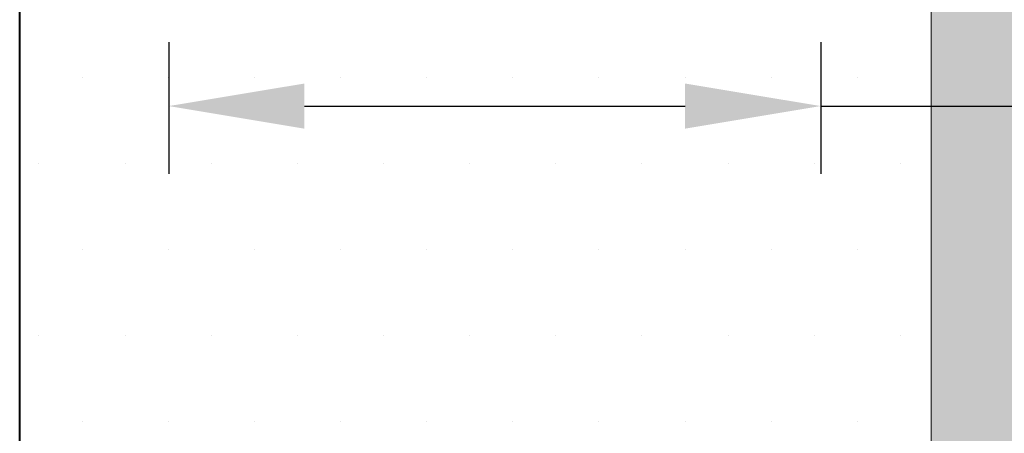
# Model space of a CAD drawing. Units: inches. Extents: x 459864 to 460310, y 324185 to 324787.
# Tile 3 of 112: x 460061 to 460079, y 324221 to 324229. Entities that reach past the tile are written whole.
import ezdxf

# ---------------------------------------------------------------- set-up
doc = ezdxf.new("R2010")
doc.units = ezdxf.units.IN
for name, color, linetype, lineweight in [('A-ANNO-DIMS', 2, 'Continuous', 18), ('A-WALL', 7, 'Continuous', 40), ('L-HRDS', 9, 'Continuous', 18), ('L-SITE-PATT', 252, 'Continuous', 13)]:
    doc.layers.add(name, color=color, linetype=linetype, lineweight=lineweight)
doc.styles.get("Standard").update_dxf_attribs({"font": 'arial.ttf'})
doc.dimstyles.new('ISO-25', dxfattribs={"dimtxt": 6, "dimasz": 2.5, "dimexe": 1.25, "dimexo": 0.625, "dimtad": 1, "dimdec": 1, "dimlunit": 3, "dimtxsty": 'Standard', "dimcen": 2.5, "dimadec": 0, "dimazin": 0, "dimtfac": 1, "dimtdec": 1, "dimtmove": 0, "dimatfit": 3, "dimfxl": 1, "dimarcsym": 0})

# ---------------------------------------------------------------- blocks, each defined once
blk = doc.blocks.new('*D36')
at = {"layer": 'A-ANNO-DIMS', "color": 0, "lineweight": -2, "transparency": 16777216}
for p, q in [((460063.861, 324228.483), (460063.861, 324226.056)), ((460075.876, 324228.483), (460075.876, 324226.056)), ((460066.361, 324227.306), (460073.376, 324227.306)), ((460075.876, 324227.306), (460126.021, 324227.306))]:
    blk.add_line(p, q, dxfattribs=at)
at = {"layer": 'A-ANNO-DIMS', "color": 0, "transparency": 16777216}
for points in [[(460066.361, 324227.722), (460066.361, 324226.889), (460063.861, 324227.306)], [(460073.376, 324227.722), (460073.376, 324226.889), (460075.876, 324227.306)]]:
    blk.add_solid(points, dxfattribs=at)
at = {"layer": 'Defpoints', "color": 0, "transparency": 16777216}
for p in [(460063.861, 324229.108), (460075.876, 324229.108), (460075.876, 324227.306)]:
    blk.add_point(p, dxfattribs=at)
at = {"layer": 'A-ANNO-DIMS', "color": 0, "transparency": 16777216, "insert": (460102.199, 324230.994), "char_height": 6, "attachment_point": 5}
blk.add_mtext('PAVER 1\'-0"', dxfattribs=at)

msp = doc.modelspace()

# ---------------------------------------------------------------- hatches: boundary and pattern name
at = {"layer": 'L-SITE-PATT'}
h = msp.add_hatch(dxfattribs=at)
h.set_pattern_fill('DOTS', color=256)
h.paths.add_polyline_path([(460269.804, 324283.483), (460247.115, 324283.483), (460121.929, 324283.483), (460121.929, 324252.473), (460117.429, 324252.473), (460110.124, 324252.473), (460110.124, 324243.287), (460080.83, 324243.287), (460080.83, 324252.473), (460061.115, 324252.473), (460061.115, 324251.882), (460077.909, 324251.882), (460077.909, 324199.483), (460080.83, 324199.483), (460080.83, 324207.553), (460110.124, 324207.553), (460110.124, 324199.483), (460110.813, 324199.483), (460262.115, 324199.483), (460269.804, 324199.483)], flags=17)
edge = h.paths.add_edge_path(flags=0)
edge.add_ellipse((460222.59, 324263.813), major_axis=(-8.485, 8.485), ratio=1, start_angle=405, end_angle=495, ccw=False)
edge.add_line((460214.821, 324254.66), (460214.832, 324254.666))
edge.add_ellipse((460222.59, 324263.813), major_axis=(-8.485, 8.485), ratio=1, start_angle=405, end_angle=495, ccw=False)
edge.add_line((460210.759, 324261.781), (460210.768, 324261.787))
edge.add_ellipse((460222.59, 324263.813), major_axis=(-8.485, 8.485), ratio=1, start_angle=405, end_angle=495, ccw=False)
edge.add_ellipse((460222.59, 324263.813), major_axis=(-8.485, 8.485), ratio=1, start_angle=392.754, end_angle=405, ccw=False)
edge.add_ellipse((460222.59, 324263.813), major_axis=(-8.485, 8.485), ratio=1, start_angle=380.9347, end_angle=392.754, ccw=False)
edge.add_line((460211.337, 324267.985), (460211.34, 324267.985))
edge.add_ellipse((460222.59, 324263.813), major_axis=(-8.485, 8.485), ratio=1, start_angle=380.9347, end_angle=392.754, ccw=False)
edge.add_ellipse((460222.59, 324263.813), major_axis=(-8.485, 8.485), ratio=1, start_angle=347.9015, end_angle=380.9347, ccw=False)
edge.add_ellipse((460222.59, 324263.813), major_axis=(-8.485, 8.485), ratio=1, start_angle=327.0619, end_angle=347.9015, ccw=False)
edge.add_ellipse((460222.59, 324263.813), major_axis=(-8.485, 8.485), ratio=1, start_angle=278.3246, end_angle=327.0619, ccw=False)
edge.add_line((460225.158, 324275.536), (460225.158, 324275.535))
edge.add_ellipse((460222.59, 324263.813), major_axis=(-8.485, 8.485), ratio=1, start_angle=278.3246, end_angle=327.0619, ccw=False)
edge.add_ellipse((460222.59, 324263.813), major_axis=(-8.485, 8.485), ratio=1, start_angle=260.6436, end_angle=278.3246, ccw=False)
edge.add_ellipse((460222.59, 324263.813), major_axis=(-8.485, 8.485), ratio=1, start_angle=225, end_angle=260.6436, ccw=False)
edge.add_line((460234.509, 324265.243), (460234.501, 324265.239))
edge.add_ellipse((460222.59, 324263.813), major_axis=(-8.485, 8.485), ratio=1, start_angle=225, end_angle=260.6436, ccw=False)
edge.add_ellipse((460222.59, 324263.813), major_axis=(-8.485, 8.485), ratio=1, start_angle=495, end_angle=585, ccw=False)
edge.add_line((460234.437, 324261.861), (460234.424, 324261.858))
edge.add_ellipse((460222.59, 324263.813), major_axis=(-8.485, 8.485), ratio=1, start_angle=495, end_angle=585, ccw=False)
edge.add_line((460227.95, 324253.067), (460227.946, 324253.083))
edge.add_ellipse((460222.59, 324263.813), major_axis=(-8.485, 8.485), ratio=1, start_angle=495, end_angle=585, ccw=False)
edge.add_line((460226.223, 324252.369), (460226.211, 324252.38))
edge.add_ellipse((460222.59, 324263.813), major_axis=(-8.485, 8.485), ratio=1, start_angle=495, end_angle=585, ccw=False)
h.paths.add_polyline_path([(460219.651, 324254.347), (460218.461, 324253.545), (460218.275, 324254.789), (460219.642, 324256.542), (460219.625, 324260.848), (460216.11, 324257.333), (460214.35, 324256.978), (460215.416, 324259.356), (460212.524, 324258.496), (460213.137, 324259.93), (460218.507, 324263.813), (460222.59, 324263.813), (460222.59, 324267.807), (460218.176, 324272.212), (460219.026, 324274.639), (460222.59, 324272.811), (460222.59, 324275.423), (460223.057, 324274.825), (460222.675, 324273.492), (460225.912, 324267.135), (460219.625, 324260.848)], flags=0)
edge = h.paths.add_edge_path(flags=0)
edge.add_ellipse((460194.576, 324264.046), major_axis=(-8.485, 8.485), ratio=1, start_angle=495, end_angle=585, ccw=False)
edge.add_line((460199.936, 324253.3), (460199.932, 324253.316))
edge.add_ellipse((460194.576, 324264.046), major_axis=(-8.485, 8.485), ratio=1, start_angle=495, end_angle=585, ccw=False)
edge.add_line((460198.208, 324252.603), (460198.196, 324252.613))
edge.add_ellipse((460194.576, 324264.046), major_axis=(-8.485, 8.485), ratio=1, start_angle=495, end_angle=585, ccw=False)
edge.add_ellipse((460194.576, 324264.046), major_axis=(-8.485, 8.485), ratio=1, start_angle=405, end_angle=495, ccw=False)
edge.add_line((460186.806, 324254.893), (460186.817, 324254.899))
edge.add_ellipse((460194.576, 324264.046), major_axis=(-8.485, 8.485), ratio=1, start_angle=405, end_angle=495, ccw=False)
edge.add_line((460182.744, 324262.014), (460182.753, 324262.02))
edge.add_ellipse((460194.576, 324264.046), major_axis=(-8.485, 8.485), ratio=1, start_angle=405, end_angle=495, ccw=False)
edge.add_ellipse((460194.576, 324264.046), major_axis=(-8.485, 8.485), ratio=1, start_angle=392.754, end_angle=405, ccw=False)
edge.add_ellipse((460194.576, 324264.046), major_axis=(-8.485, 8.485), ratio=1, start_angle=380.9347, end_angle=392.754, ccw=False)
edge.add_line((460183.323, 324268.218), (460183.326, 324268.218))
edge.add_ellipse((460194.576, 324264.046), major_axis=(-8.485, 8.485), ratio=1, start_angle=380.9347, end_angle=392.754, ccw=False)
edge.add_ellipse((460194.576, 324264.046), major_axis=(-8.485, 8.485), ratio=1, start_angle=347.9015, end_angle=380.9347, ccw=False)
edge.add_ellipse((460194.576, 324264.046), major_axis=(-8.485, 8.485), ratio=1, start_angle=327.0619, end_angle=347.9015, ccw=False)
edge.add_ellipse((460194.576, 324264.046), major_axis=(-8.485, 8.485), ratio=1, start_angle=278.3246, end_angle=327.0619, ccw=False)
edge.add_line((460197.144, 324275.769), (460197.143, 324275.768))
edge.add_ellipse((460194.576, 324264.046), major_axis=(-8.485, 8.485), ratio=1, start_angle=278.3246, end_angle=327.0619, ccw=False)
edge.add_ellipse((460194.576, 324264.046), major_axis=(-8.485, 8.485), ratio=1, start_angle=260.6436, end_angle=278.3246, ccw=False)
edge.add_ellipse((460194.576, 324264.046), major_axis=(-8.485, 8.485), ratio=1, start_angle=225, end_angle=260.6436, ccw=False)
edge.add_line((460206.494, 324265.476), (460206.487, 324265.473))
edge.add_ellipse((460194.576, 324264.046), major_axis=(-8.485, 8.485), ratio=1, start_angle=225, end_angle=260.6436, ccw=False)
edge.add_ellipse((460194.576, 324264.046), major_axis=(-8.485, 8.485), ratio=1, start_angle=495, end_angle=585, ccw=False)
edge.add_line((460206.422, 324262.094), (460206.409, 324262.091))
h.paths.add_polyline_path([(460191.61, 324261.081), (460191.637, 324254.58), (460190.447, 324253.778), (460190.261, 324255.023), (460191.628, 324256.775), (460191.61, 324261.081), (460188.096, 324257.566), (460186.335, 324257.211), (460187.402, 324259.589), (460184.509, 324258.729), (460185.123, 324260.163), (460190.493, 324264.046), (460194.576, 324264.046), (460194.576, 324268.04), (460190.161, 324272.446), (460191.011, 324274.872), (460194.576, 324273.044), (460194.576, 324275.657), (460195.043, 324275.058), (460194.661, 324273.725), (460197.897, 324267.368)], flags=0)
edge = h.paths.add_edge_path(flags=0)
edge.add_ellipse((460252.912, 324263.578), major_axis=(-8.485, 8.485), ratio=1, start_angle=405, end_angle=495, ccw=False)
edge.add_line((460241.081, 324261.545), (460241.089, 324261.551))
edge.add_ellipse((460252.912, 324263.578), major_axis=(-8.485, 8.485), ratio=1, start_angle=405, end_angle=495, ccw=False)
edge.add_ellipse((460252.912, 324263.578), major_axis=(-8.485, 8.485), ratio=1, start_angle=392.754, end_angle=405, ccw=False)
edge.add_ellipse((460252.912, 324263.578), major_axis=(-8.485, 8.485), ratio=1, start_angle=380.9347, end_angle=392.754, ccw=False)
edge.add_line((460241.659, 324267.749), (460241.662, 324267.749))
edge.add_ellipse((460252.912, 324263.578), major_axis=(-8.485, 8.485), ratio=1, start_angle=380.9347, end_angle=392.754, ccw=False)
edge.add_ellipse((460252.912, 324263.578), major_axis=(-8.485, 8.485), ratio=1, start_angle=347.9015, end_angle=380.9347, ccw=False)
edge.add_ellipse((460252.912, 324263.578), major_axis=(-8.485, 8.485), ratio=1, start_angle=327.0619, end_angle=347.9015, ccw=False)
edge.add_ellipse((460252.912, 324263.578), major_axis=(-8.485, 8.485), ratio=1, start_angle=278.3246, end_angle=327.0619, ccw=False)
edge.add_line((460255.48, 324275.3), (460255.479, 324275.299))
edge.add_ellipse((460252.912, 324263.578), major_axis=(-8.485, 8.485), ratio=1, start_angle=278.3246, end_angle=327.0619, ccw=False)
edge.add_ellipse((460252.912, 324263.578), major_axis=(-8.485, 8.485), ratio=1, start_angle=260.6436, end_angle=278.3246, ccw=False)
edge.add_ellipse((460252.912, 324263.578), major_axis=(-8.485, 8.485), ratio=1, start_angle=225, end_angle=260.6436, ccw=False)
edge.add_line((460264.83, 324265.007), (460264.823, 324265.004))
edge.add_ellipse((460252.912, 324263.578), major_axis=(-8.485, 8.485), ratio=1, start_angle=225, end_angle=260.6436, ccw=False)
edge.add_ellipse((460252.912, 324263.578), major_axis=(-8.485, 8.485), ratio=1, start_angle=495, end_angle=585, ccw=False)
edge.add_line((460264.758, 324261.626), (460264.745, 324261.622))
edge.add_ellipse((460252.912, 324263.578), major_axis=(-8.485, 8.485), ratio=1, start_angle=495, end_angle=585, ccw=False)
edge.add_line((460258.272, 324252.832), (460258.268, 324252.848))
edge.add_ellipse((460252.912, 324263.578), major_axis=(-8.485, 8.485), ratio=1, start_angle=495, end_angle=585, ccw=False)
edge.add_line((460256.545, 324252.134), (460256.533, 324252.144))
edge.add_ellipse((460252.912, 324263.578), major_axis=(-8.485, 8.485), ratio=1, start_angle=495, end_angle=585, ccw=False)
edge.add_ellipse((460252.912, 324263.578), major_axis=(-8.485, 8.485), ratio=1, start_angle=405, end_angle=495, ccw=False)
edge.add_line((460245.143, 324254.424), (460245.153, 324254.43))
h.paths.add_polyline_path([(460244.672, 324256.742), (460245.738, 324259.12), (460242.846, 324258.26), (460243.459, 324259.694), (460248.829, 324263.578), (460252.912, 324263.578), (460252.912, 324267.571), (460248.497, 324271.977), (460249.348, 324274.403), (460252.912, 324272.576), (460252.912, 324275.188), (460253.379, 324274.589), (460252.997, 324273.257), (460256.233, 324266.899), (460249.946, 324260.612), (460249.973, 324254.111), (460248.783, 324253.309), (460248.597, 324254.554), (460249.964, 324256.306), (460249.946, 324260.612), (460246.432, 324257.097)], flags=0)
edge = h.paths.add_edge_path(flags=0)
edge.add_ellipse((460167.439, 324262.833), major_axis=(-8.485, 8.485), ratio=1, start_angle=495, end_angle=585, ccw=False)
edge.add_line((460172.799, 324252.087), (460172.795, 324252.103))
edge.add_ellipse((460167.439, 324262.833), major_axis=(-8.485, 8.485), ratio=1, start_angle=495, end_angle=585, ccw=False)
edge.add_line((460171.071, 324251.389), (460171.059, 324251.399))
edge.add_ellipse((460167.439, 324262.833), major_axis=(-8.485, 8.485), ratio=1, start_angle=495, end_angle=585, ccw=False)
edge.add_ellipse((460167.439, 324262.833), major_axis=(-8.485, 8.485), ratio=1, start_angle=405, end_angle=495, ccw=False)
edge.add_line((460159.669, 324253.679), (460159.68, 324253.685))
edge.add_ellipse((460167.439, 324262.833), major_axis=(-8.485, 8.485), ratio=1, start_angle=405, end_angle=495, ccw=False)
edge.add_line((460155.607, 324260.8), (460155.616, 324260.806))
edge.add_ellipse((460167.439, 324262.833), major_axis=(-8.485, 8.485), ratio=1, start_angle=405, end_angle=495, ccw=False)
edge.add_ellipse((460167.439, 324262.833), major_axis=(-8.485, 8.485), ratio=1, start_angle=392.754, end_angle=405, ccw=False)
edge.add_ellipse((460167.439, 324262.833), major_axis=(-8.485, 8.485), ratio=1, start_angle=380.9347, end_angle=392.754, ccw=False)
edge.add_line((460156.185, 324267.005), (460156.189, 324267.005))
edge.add_ellipse((460167.439, 324262.833), major_axis=(-8.485, 8.485), ratio=1, start_angle=380.9347, end_angle=392.754, ccw=False)
edge.add_ellipse((460167.439, 324262.833), major_axis=(-8.485, 8.485), ratio=1, start_angle=347.9015, end_angle=380.9347, ccw=False)
edge.add_ellipse((460167.439, 324262.833), major_axis=(-8.485, 8.485), ratio=1, start_angle=327.0619, end_angle=347.9015, ccw=False)
edge.add_ellipse((460167.439, 324262.833), major_axis=(-8.485, 8.485), ratio=1, start_angle=278.3246, end_angle=327.0619, ccw=False)
edge.add_line((460170.007, 324274.556), (460170.006, 324274.554))
edge.add_ellipse((460167.439, 324262.833), major_axis=(-8.485, 8.485), ratio=1, start_angle=278.3246, end_angle=327.0619, ccw=False)
edge.add_ellipse((460167.439, 324262.833), major_axis=(-8.485, 8.485), ratio=1, start_angle=260.6436, end_angle=278.3246, ccw=False)
edge.add_ellipse((460167.439, 324262.833), major_axis=(-8.485, 8.485), ratio=1, start_angle=225, end_angle=260.6436, ccw=False)
edge.add_line((460179.357, 324264.262), (460179.35, 324264.259))
edge.add_ellipse((460167.439, 324262.833), major_axis=(-8.485, 8.485), ratio=1, start_angle=225, end_angle=260.6436, ccw=False)
edge.add_ellipse((460167.439, 324262.833), major_axis=(-8.485, 8.485), ratio=1, start_angle=495, end_angle=585, ccw=False)
edge.add_line((460179.285, 324260.881), (460179.272, 324260.877))
h.paths.add_polyline_path([(460164.473, 324259.867), (460164.5, 324253.366), (460163.31, 324252.565), (460163.124, 324253.809), (460164.491, 324255.561), (460164.473, 324259.867), (460160.958, 324256.353), (460159.198, 324255.998), (460160.265, 324258.375), (460157.372, 324257.515), (460157.986, 324258.949), (460163.356, 324262.833), (460167.439, 324262.833), (460167.439, 324266.826), (460163.024, 324271.232), (460163.874, 324273.659), (460167.439, 324271.831), (460167.439, 324274.443), (460167.905, 324273.844), (460167.524, 324272.512), (460170.76, 324266.154)], flags=0)
edge = h.paths.add_edge_path(flags=0)
edge.add_ellipse((460140.758, 324262.37), major_axis=(-8.485, 8.485), ratio=1, start_angle=495, end_angle=585, ccw=False)
edge.add_line((460146.118, 324251.624), (460146.114, 324251.639))
edge.add_ellipse((460140.758, 324262.37), major_axis=(-8.485, 8.485), ratio=1, start_angle=495, end_angle=585, ccw=False)
edge.add_line((460144.391, 324250.926), (460144.379, 324250.936))
edge.add_ellipse((460140.758, 324262.37), major_axis=(-8.485, 8.485), ratio=1, start_angle=495, end_angle=585, ccw=False)
edge.add_ellipse((460140.758, 324262.37), major_axis=(-8.485, 8.485), ratio=1, start_angle=405, end_angle=495, ccw=False)
edge.add_line((460132.989, 324253.216), (460132.999, 324253.222))
edge.add_ellipse((460140.758, 324262.37), major_axis=(-8.485, 8.485), ratio=1, start_angle=405, end_angle=495, ccw=False)
edge.add_line((460128.927, 324260.337), (460128.935, 324260.343))
edge.add_ellipse((460140.758, 324262.37), major_axis=(-8.485, 8.485), ratio=1, start_angle=405, end_angle=495, ccw=False)
edge.add_ellipse((460140.758, 324262.37), major_axis=(-8.485, 8.485), ratio=1, start_angle=392.754, end_angle=405, ccw=False)
edge.add_ellipse((460140.758, 324262.37), major_axis=(-8.485, 8.485), ratio=1, start_angle=380.9347, end_angle=392.754, ccw=False)
edge.add_line((460129.505, 324266.541), (460129.508, 324266.541))
edge.add_ellipse((460140.758, 324262.37), major_axis=(-8.485, 8.485), ratio=1, start_angle=380.9347, end_angle=392.754, ccw=False)
edge.add_ellipse((460140.758, 324262.37), major_axis=(-8.485, 8.485), ratio=1, start_angle=347.9015, end_angle=380.9347, ccw=False)
edge.add_ellipse((460140.758, 324262.37), major_axis=(-8.485, 8.485), ratio=1, start_angle=327.0619, end_angle=347.9015, ccw=False)
edge.add_ellipse((460140.758, 324262.37), major_axis=(-8.485, 8.485), ratio=1, start_angle=278.3246, end_angle=327.0619, ccw=False)
edge.add_line((460143.326, 324274.092), (460143.325, 324274.091))
edge.add_ellipse((460140.758, 324262.37), major_axis=(-8.485, 8.485), ratio=1, start_angle=278.3246, end_angle=327.0619, ccw=False)
edge.add_ellipse((460140.758, 324262.37), major_axis=(-8.485, 8.485), ratio=1, start_angle=260.6436, end_angle=278.3246, ccw=False)
edge.add_ellipse((460140.758, 324262.37), major_axis=(-8.485, 8.485), ratio=1, start_angle=225, end_angle=260.6436, ccw=False)
edge.add_line((460152.677, 324263.799), (460152.669, 324263.796))
edge.add_ellipse((460140.758, 324262.37), major_axis=(-8.485, 8.485), ratio=1, start_angle=225, end_angle=260.6436, ccw=False)
edge.add_ellipse((460140.758, 324262.37), major_axis=(-8.485, 8.485), ratio=1, start_angle=495, end_angle=585, ccw=False)
edge.add_line((460152.604, 324260.418), (460152.592, 324260.414))
h.paths.add_polyline_path([(460137.792, 324259.404), (460137.819, 324252.903), (460136.629, 324252.101), (460136.443, 324253.346), (460137.81, 324255.098), (460137.792, 324259.404), (460134.278, 324255.889), (460132.518, 324255.534), (460133.584, 324257.912), (460130.692, 324257.052), (460131.305, 324258.486), (460136.675, 324262.37), (460140.758, 324262.37), (460140.758, 324266.363), (460136.343, 324270.769), (460137.194, 324273.195), (460140.758, 324271.367), (460140.758, 324273.98), (460141.225, 324273.381), (460140.843, 324272.049), (460144.079, 324265.691)], flags=0)
h.paths.add_polyline_path([(460110.124, 324227.414), (460080.83, 324227.414), (460080.83, 324235.484), (460110.124, 324235.484)], flags=16)
h.paths.add_polyline_path([(460110.124, 324220.797), (460110.124, 324212.727), (460080.83, 324212.727), (460080.83, 324220.797)], flags=16)
h.paths.add_polyline_path([(460269.804, 324283.483), (460247.115, 324283.483), (460121.929, 324283.483), (460121.929, 324252.473), (460117.429, 324252.473), (460110.124, 324252.473), (460110.124, 324243.287), (460080.83, 324243.287), (460080.83, 324252.473), (460061.115, 324252.473), (460061.115, 324251.882), (460077.909, 324251.882), (460077.909, 324199.483), (460080.83, 324199.483), (460080.83, 324207.553), (460110.124, 324207.553), (460110.124, 324199.483), (460262.115, 324199.483), (460269.804, 324199.483)], flags=17)
h.paths.add_polyline_path([(460219.651, 324254.347), (460218.461, 324253.545), (460218.275, 324254.789), (460219.642, 324256.542), (460219.625, 324260.848), (460216.11, 324257.333), (460214.35, 324256.978), (460215.416, 324259.356), (460212.524, 324258.496), (460213.137, 324259.93), (460218.507, 324263.813), (460222.59, 324263.813), (460220.18, 324266.223), (460215.461, 324265.308), (460211.835, 324266.137), (460216.247, 324267.985), (460218.418, 324267.985), (460222.59, 324263.813), (460222.59, 324267.807), (460218.176, 324272.212), (460219.026, 324274.639), (460222.59, 324272.811), (460222.59, 324275.423), (460223.057, 324274.825), (460222.675, 324273.492), (460225.912, 324267.135), (460222.59, 324263.813), (460231.383, 324263.813), (460228.485, 324262.488), (460224.425, 324261.978), (460228.68, 324257.724), (460228.966, 324254.791), (460227.142, 324256.537), (460227.542, 324254.819), (460227.333, 324253.614), (460222.59, 324259.985), (460222.59, 324255.497), (460221.377, 324256.541), (460220.576, 324261.799), (460219.625, 324260.848)], flags=0)
h.paths.add_polyline_path([(460199.127, 324256.77), (460199.528, 324255.052), (460199.319, 324253.848), (460194.576, 324260.218), (460194.576, 324255.73), (460193.363, 324256.774), (460192.561, 324262.032), (460191.61, 324261.081), (460191.637, 324254.58), (460190.447, 324253.778), (460190.261, 324255.023), (460191.628, 324256.775), (460191.61, 324261.081), (460188.096, 324257.566), (460186.335, 324257.211), (460187.402, 324259.589), (460184.509, 324258.729), (460185.123, 324260.163), (460190.493, 324264.046), (460194.576, 324264.046), (460192.166, 324266.456), (460187.446, 324265.541), (460183.82, 324266.37), (460188.232, 324268.218), (460190.404, 324268.218), (460194.576, 324264.046), (460194.576, 324268.04), (460190.161, 324272.446), (460191.011, 324274.872), (460194.576, 324273.044), (460194.576, 324275.657), (460195.043, 324275.058), (460194.661, 324273.725), (460197.897, 324267.368), (460194.576, 324264.046), (460203.368, 324264.046), (460200.47, 324262.721), (460196.411, 324262.212), (460200.665, 324257.957), (460200.951, 324255.024)], flags=0)
h.paths.add_polyline_path([(460244.672, 324256.742), (460245.738, 324259.12), (460242.846, 324258.26), (460243.459, 324259.694), (460248.829, 324263.578), (460252.912, 324263.578), (460250.502, 324265.987), (460245.783, 324265.072), (460242.156, 324265.901), (460246.568, 324267.749), (460248.74, 324267.749), (460252.912, 324263.578), (460252.912, 324267.571), (460248.497, 324271.977), (460249.348, 324274.403), (460252.912, 324272.576), (460252.912, 324275.188), (460253.379, 324274.589), (460252.997, 324273.257), (460256.233, 324266.899), (460252.912, 324263.578), (460261.705, 324263.578), (460258.806, 324262.252), (460254.747, 324261.743), (460259.002, 324257.488), (460259.288, 324254.555), (460257.463, 324256.301), (460257.864, 324254.583), (460257.655, 324253.379), (460252.912, 324259.749), (460252.912, 324255.261), (460251.699, 324256.305), (460250.897, 324261.563), (460249.946, 324260.612), (460249.973, 324254.111), (460248.783, 324253.309), (460248.597, 324254.554), (460249.964, 324256.306), (460249.946, 324260.612), (460246.432, 324257.097)], flags=0)
h.paths.add_polyline_path([(460173.528, 324256.743), (460173.814, 324253.811), (460171.99, 324255.556), (460172.39, 324253.838), (460172.182, 324252.634), (460167.439, 324259.004), (460167.439, 324254.516), (460166.226, 324255.56), (460165.424, 324260.818), (460164.473, 324259.867), (460164.5, 324253.366), (460163.31, 324252.565), (460163.124, 324253.809), (460164.491, 324255.561), (460164.473, 324259.867), (460160.958, 324256.353), (460159.198, 324255.998), (460160.265, 324258.375), (460157.372, 324257.515), (460157.986, 324258.949), (460163.356, 324262.833), (460167.439, 324262.833), (460165.029, 324265.243), (460160.309, 324264.327), (460156.683, 324265.156), (460161.095, 324267.005), (460163.267, 324267.005), (460167.439, 324262.833), (460167.439, 324266.826), (460163.024, 324271.232), (460163.874, 324273.659), (460167.439, 324271.831), (460167.439, 324274.443), (460167.905, 324273.844), (460167.524, 324272.512), (460170.76, 324266.154), (460167.439, 324262.833), (460176.231, 324262.833), (460173.333, 324261.507), (460169.274, 324260.998)], flags=0)
h.paths.add_polyline_path([(460146.848, 324256.28), (460147.134, 324253.347), (460145.31, 324255.093), (460145.71, 324253.375), (460145.501, 324252.171), (460140.758, 324258.541), (460140.758, 324254.053), (460139.545, 324255.097), (460138.744, 324260.355), (460137.792, 324259.404), (460137.819, 324252.903), (460136.629, 324252.101), (460136.443, 324253.346), (460137.81, 324255.098), (460137.792, 324259.404), (460134.278, 324255.889), (460132.518, 324255.534), (460133.584, 324257.912), (460130.692, 324257.052), (460131.305, 324258.486), (460136.675, 324262.37), (460140.758, 324262.37), (460138.348, 324264.779), (460133.629, 324263.864), (460130.002, 324264.693), (460134.414, 324266.541), (460136.586, 324266.541), (460140.758, 324262.37), (460140.758, 324266.363), (460136.343, 324270.769), (460137.194, 324273.195), (460140.758, 324271.367), (460140.758, 324273.98), (460141.225, 324273.381), (460140.843, 324272.049), (460144.079, 324265.691), (460140.758, 324262.37), (460149.551, 324262.37), (460146.653, 324261.044), (460142.593, 324260.535)], flags=0)
edge = h.paths.add_edge_path()
edge.add_line((460269.804, 324272.549), (460260.881, 324272.549))
edge.add_ellipse((460252.912, 324263.578), major_axis=(-8.485, 8.485), ratio=1, start_angle=260.6436, end_angle=273.3846, ccw=False)
edge.add_line((460262.283, 324271.092), (460262.261, 324271.091))
edge.add_ellipse((460252.912, 324263.578), major_axis=(-8.485, 8.485), ratio=1, start_angle=260.6436, end_angle=273.3846, ccw=False)
edge.add_ellipse((460252.912, 324263.578), major_axis=(-8.485, 8.485), ratio=1, start_angle=225, end_angle=260.6436, ccw=False)
edge.add_line((460263.609, 324269.063), (460263.572, 324269.058))
edge.add_ellipse((460252.912, 324263.578), major_axis=(-8.485, 8.485), ratio=1, start_angle=225, end_angle=260.6436, ccw=False)
edge.add_line((460264.615, 324266.306), (460264.585, 324266.305))
edge.add_ellipse((460252.912, 324263.578), major_axis=(-8.485, 8.485), ratio=1, start_angle=225, end_angle=260.6436, ccw=False)
edge.add_line((460264.83, 324265.007), (460264.823, 324265.004))
edge.add_ellipse((460252.912, 324263.578), major_axis=(-8.485, 8.485), ratio=1, start_angle=225, end_angle=260.6436, ccw=False)
edge.add_ellipse((460252.912, 324263.578), major_axis=(-8.485, 8.485), ratio=1, start_angle=495, end_angle=585, ccw=False)
edge.add_line((460264.758, 324261.626), (460264.745, 324261.622))
edge.add_ellipse((460252.912, 324263.578), major_axis=(-8.485, 8.485), ratio=1, start_angle=495, end_angle=585, ccw=False)
edge.add_line((460263.442, 324257.739), (460263.389, 324257.779))
edge.add_ellipse((460252.912, 324263.578), major_axis=(-8.485, 8.485), ratio=1, start_angle=495, end_angle=585, ccw=False)
edge.add_line((460258.128, 324252.744), (460258.102, 324252.779))
edge.add_ellipse((460252.912, 324263.578), major_axis=(-8.485, 8.485), ratio=1, start_angle=495, end_angle=585, ccw=False)
edge.add_line((460256.545, 324252.134), (460256.533, 324252.144))
edge.add_ellipse((460252.912, 324263.578), major_axis=(-8.485, 8.485), ratio=1, start_angle=495, end_angle=585, ccw=False)
edge.add_ellipse((460252.912, 324263.578), major_axis=(-8.485, 8.485), ratio=1, start_angle=405, end_angle=495, ccw=False)
edge.add_line((460250.594, 324251.78), (460250.605, 324251.82))
edge.add_ellipse((460252.912, 324263.578), major_axis=(-8.485, 8.485), ratio=1, start_angle=405, end_angle=495, ccw=False)
edge.add_line((460245.143, 324254.424), (460245.153, 324254.43))
edge.add_ellipse((460252.912, 324263.578), major_axis=(-8.485, 8.485), ratio=1, start_angle=405, end_angle=495, ccw=False)
edge.add_line((460243.525, 324256.059), (460243.56, 324256.091))
edge.add_ellipse((460252.912, 324263.578), major_axis=(-8.485, 8.485), ratio=1, start_angle=405, end_angle=495, ccw=False)
edge.add_line((460241.44, 324259.893), (460241.522, 324259.896))
edge.add_ellipse((460252.912, 324263.578), major_axis=(-8.485, 8.485), ratio=1, start_angle=405, end_angle=495, ccw=False)
edge.add_line((460241.081, 324261.545), (460241.089, 324261.551))
edge.add_ellipse((460252.912, 324263.578), major_axis=(-8.485, 8.485), ratio=1, start_angle=405, end_angle=495, ccw=False)
edge.add_ellipse((460252.912, 324263.578), major_axis=(-8.485, 8.485), ratio=1, start_angle=392.754, end_angle=405, ccw=False)
edge.add_line((460241.05, 324265.438), (460241.063, 324265.443))
edge.add_ellipse((460252.912, 324263.578), major_axis=(-8.485, 8.485), ratio=1, start_angle=392.754, end_angle=405, ccw=False)
edge.add_ellipse((460252.912, 324263.578), major_axis=(-8.485, 8.485), ratio=1, start_angle=380.9347, end_angle=392.754, ccw=False)
edge.add_line((460241.452, 324267.176), (460241.469, 324267.171))
edge.add_ellipse((460252.912, 324263.578), major_axis=(-8.485, 8.485), ratio=1, start_angle=380.9347, end_angle=392.754, ccw=False)
edge.add_line((460241.659, 324267.749), (460241.662, 324267.749))
edge.add_ellipse((460252.912, 324263.578), major_axis=(-8.485, 8.485), ratio=1, start_angle=380.9347, end_angle=392.754, ccw=False)
edge.add_ellipse((460252.912, 324263.578), major_axis=(-8.485, 8.485), ratio=1, start_angle=356.6154, end_angle=380.9347, ccw=False)
edge.add_line((460244.88, 324272.488), (460244.713, 324272.549))
edge.add_line((460244.713, 324272.549), (460230.817, 324272.549))
edge.add_ellipse((460222.59, 324263.813), major_axis=(-8.485, 8.485), ratio=1, start_angle=260.6436, end_angle=271.7178, ccw=False)
edge.add_ellipse((460222.59, 324263.813), major_axis=(-8.485, 8.485), ratio=1, start_angle=225, end_angle=260.6436, ccw=False)
edge.add_line((460233.287, 324269.299), (460233.25, 324269.294))
edge.add_ellipse((460222.59, 324263.813), major_axis=(-8.485, 8.485), ratio=1, start_angle=225, end_angle=260.6436, ccw=False)
edge.add_line((460234.294, 324266.541), (460234.264, 324266.541))
edge.add_ellipse((460222.59, 324263.813), major_axis=(-8.485, 8.485), ratio=1, start_angle=225, end_angle=260.6436, ccw=False)
edge.add_line((460234.509, 324265.243), (460234.501, 324265.239))
edge.add_ellipse((460222.59, 324263.813), major_axis=(-8.485, 8.485), ratio=1, start_angle=225, end_angle=260.6436, ccw=False)
edge.add_ellipse((460222.59, 324263.813), major_axis=(-8.485, 8.485), ratio=1, start_angle=495, end_angle=585, ccw=False)
edge.add_line((460234.437, 324261.861), (460234.424, 324261.858))
edge.add_ellipse((460222.59, 324263.813), major_axis=(-8.485, 8.485), ratio=1, start_angle=495, end_angle=585, ccw=False)
edge.add_line((460233.121, 324257.975), (460233.068, 324258.015))
edge.add_ellipse((460222.59, 324263.813), major_axis=(-8.485, 8.485), ratio=1, start_angle=495, end_angle=585, ccw=False)
edge.add_line((460227.806, 324252.979), (460227.78, 324253.014))
edge.add_ellipse((460222.59, 324263.813), major_axis=(-8.485, 8.485), ratio=1, start_angle=495, end_angle=585, ccw=False)
edge.add_line((460226.223, 324252.369), (460226.211, 324252.38))
edge.add_ellipse((460222.59, 324263.813), major_axis=(-8.485, 8.485), ratio=1, start_angle=495, end_angle=585, ccw=False)
edge.add_ellipse((460222.59, 324263.813), major_axis=(-8.485, 8.485), ratio=1, start_angle=405, end_angle=495, ccw=False)
edge.add_line((460220.272, 324252.016), (460220.283, 324252.055))
edge.add_ellipse((460222.59, 324263.813), major_axis=(-8.485, 8.485), ratio=1, start_angle=405, end_angle=495, ccw=False)
edge.add_line((460214.821, 324254.66), (460214.832, 324254.666))
edge.add_ellipse((460222.59, 324263.813), major_axis=(-8.485, 8.485), ratio=1, start_angle=405, end_angle=495, ccw=False)
edge.add_line((460213.203, 324256.295), (460213.239, 324256.327))
edge.add_ellipse((460222.59, 324263.813), major_axis=(-8.485, 8.485), ratio=1, start_angle=405, end_angle=495, ccw=False)
edge.add_line((460211.118, 324260.128), (460211.201, 324260.131))
edge.add_ellipse((460222.59, 324263.813), major_axis=(-8.485, 8.485), ratio=1, start_angle=405, end_angle=495, ccw=False)
edge.add_line((460210.759, 324261.781), (460210.768, 324261.787))
edge.add_ellipse((460222.59, 324263.813), major_axis=(-8.485, 8.485), ratio=1, start_angle=405, end_angle=495, ccw=False)
edge.add_ellipse((460222.59, 324263.813), major_axis=(-8.485, 8.485), ratio=1, start_angle=392.754, end_angle=405, ccw=False)
edge.add_line((460210.729, 324265.673), (460210.741, 324265.678))
edge.add_ellipse((460222.59, 324263.813), major_axis=(-8.485, 8.485), ratio=1, start_angle=392.754, end_angle=405, ccw=False)
edge.add_ellipse((460222.59, 324263.813), major_axis=(-8.485, 8.485), ratio=1, start_angle=380.9347, end_angle=392.754, ccw=False)
edge.add_line((460211.13, 324267.412), (460211.147, 324267.407))
edge.add_ellipse((460222.59, 324263.813), major_axis=(-8.485, 8.485), ratio=1, start_angle=380.9347, end_angle=392.754, ccw=False)
edge.add_line((460211.337, 324267.985), (460211.34, 324267.985))
edge.add_ellipse((460222.59, 324263.813), major_axis=(-8.485, 8.485), ratio=1, start_angle=380.9347, end_angle=392.754, ccw=False)
edge.add_ellipse((460222.59, 324263.813), major_axis=(-8.485, 8.485), ratio=1, start_angle=358.2822, end_angle=380.9347, ccw=False)
edge.add_line((460213.705, 324271.902), (460213.709, 324271.869))
edge.add_ellipse((460222.59, 324263.813), major_axis=(-8.485, 8.485), ratio=1, start_angle=358.2822, end_angle=380.9347, ccw=False)
edge.add_line((460214.363, 324272.549), (460203.078, 324272.549))
edge.add_line((460203.078, 324272.549), (460203.06, 324272.531))
edge.add_ellipse((460194.576, 324264.046), major_axis=(-8.485, 8.485), ratio=1, start_angle=260.6436, end_angle=270.1168, ccw=False)
edge.add_line((460203.957, 324271.561), (460203.921, 324271.56))
edge.add_ellipse((460194.576, 324264.046), major_axis=(-8.485, 8.485), ratio=1, start_angle=260.6436, end_angle=270.1168, ccw=False)
edge.add_ellipse((460194.576, 324264.046), major_axis=(-8.485, 8.485), ratio=1, start_angle=225, end_angle=260.6436, ccw=False)
edge.add_line((460205.272, 324269.532), (460205.235, 324269.527))
edge.add_ellipse((460194.576, 324264.046), major_axis=(-8.485, 8.485), ratio=1, start_angle=225, end_angle=260.6436, ccw=False)
edge.add_line((460206.279, 324266.774), (460206.249, 324266.774))
edge.add_ellipse((460194.576, 324264.046), major_axis=(-8.485, 8.485), ratio=1, start_angle=225, end_angle=260.6436, ccw=False)
edge.add_line((460206.494, 324265.476), (460206.487, 324265.473))
edge.add_ellipse((460194.576, 324264.046), major_axis=(-8.485, 8.485), ratio=1, start_angle=225, end_angle=260.6436, ccw=False)
edge.add_ellipse((460194.576, 324264.046), major_axis=(-8.485, 8.485), ratio=1, start_angle=495, end_angle=585, ccw=False)
edge.add_line((460206.422, 324262.094), (460206.409, 324262.091))
edge.add_ellipse((460194.576, 324264.046), major_axis=(-8.485, 8.485), ratio=1, start_angle=495, end_angle=585, ccw=False)
edge.add_line((460205.106, 324258.208), (460205.053, 324258.248))
edge.add_ellipse((460194.576, 324264.046), major_axis=(-8.485, 8.485), ratio=1, start_angle=495, end_angle=585, ccw=False)
edge.add_line((460199.792, 324253.212), (460199.766, 324253.248))
edge.add_ellipse((460194.576, 324264.046), major_axis=(-8.485, 8.485), ratio=1, start_angle=495, end_angle=585, ccw=False)
edge.add_line((460198.208, 324252.603), (460198.196, 324252.613))
edge.add_ellipse((460194.576, 324264.046), major_axis=(-8.485, 8.485), ratio=1, start_angle=495, end_angle=585, ccw=False)
edge.add_ellipse((460194.576, 324264.046), major_axis=(-8.485, 8.485), ratio=1, start_angle=405, end_angle=495, ccw=False)
edge.add_line((460192.258, 324252.249), (460192.268, 324252.289))
edge.add_ellipse((460194.576, 324264.046), major_axis=(-8.485, 8.485), ratio=1, start_angle=405, end_angle=495, ccw=False)
edge.add_line((460186.806, 324254.893), (460186.817, 324254.899))
edge.add_ellipse((460194.576, 324264.046), major_axis=(-8.485, 8.485), ratio=1, start_angle=405, end_angle=495, ccw=False)
edge.add_line((460185.188, 324256.528), (460185.224, 324256.56))
edge.add_ellipse((460194.576, 324264.046), major_axis=(-8.485, 8.485), ratio=1, start_angle=405, end_angle=495, ccw=False)
edge.add_line((460183.104, 324260.362), (460183.186, 324260.365))
edge.add_ellipse((460194.576, 324264.046), major_axis=(-8.485, 8.485), ratio=1, start_angle=405, end_angle=495, ccw=False)
edge.add_line((460182.744, 324262.014), (460182.753, 324262.02))
edge.add_ellipse((460194.576, 324264.046), major_axis=(-8.485, 8.485), ratio=1, start_angle=405, end_angle=495, ccw=False)
edge.add_ellipse((460194.576, 324264.046), major_axis=(-8.485, 8.485), ratio=1, start_angle=392.754, end_angle=405, ccw=False)
edge.add_line((460182.714, 324265.906), (460182.726, 324265.912))
edge.add_ellipse((460194.576, 324264.046), major_axis=(-8.485, 8.485), ratio=1, start_angle=392.754, end_angle=405, ccw=False)
edge.add_ellipse((460194.576, 324264.046), major_axis=(-8.485, 8.485), ratio=1, start_angle=380.9347, end_angle=392.754, ccw=False)
edge.add_line((460183.116, 324267.645), (460183.133, 324267.64))
edge.add_ellipse((460194.576, 324264.046), major_axis=(-8.485, 8.485), ratio=1, start_angle=380.9347, end_angle=392.754, ccw=False)
edge.add_line((460183.323, 324268.218), (460183.326, 324268.218))
edge.add_ellipse((460194.576, 324264.046), major_axis=(-8.485, 8.485), ratio=1, start_angle=380.9347, end_angle=392.754, ccw=False)
edge.add_ellipse((460194.576, 324264.046), major_axis=(-8.485, 8.485), ratio=1, start_angle=359.8832, end_angle=380.9347, ccw=False)
edge.add_line((460184.491, 324270.611), (460184.553, 324270.611))
edge.add_ellipse((460194.576, 324264.046), major_axis=(-8.485, 8.485), ratio=1, start_angle=359.8832, end_angle=380.9347, ccw=False)
edge.add_line((460185.346, 324271.76), (460185.379, 324271.728))
edge.add_ellipse((460194.576, 324264.046), major_axis=(-8.485, 8.485), ratio=1, start_angle=359.8832, end_angle=380.9347, ccw=False)
edge.add_line((460185.697, 324272.086), (460185.633, 324272.549))
edge.add_line((460185.633, 324272.549), (460174.683, 324272.549))
edge.add_line((460174.683, 324272.549), (460174.606, 324272.457))
edge.add_ellipse((460167.439, 324262.833), major_axis=(-8.485, 8.485), ratio=1, start_angle=260.6436, end_angle=278.3246, ccw=False)
edge.add_ellipse((460167.439, 324262.833), major_axis=(-8.485, 8.485), ratio=1, start_angle=225, end_angle=260.6436, ccw=False)
edge.add_line((460178.135, 324268.318), (460178.098, 324268.313))
edge.add_ellipse((460167.439, 324262.833), major_axis=(-8.485, 8.485), ratio=1, start_angle=225, end_angle=260.6436, ccw=False)
edge.add_line((460179.142, 324265.561), (460179.112, 324265.56))
edge.add_ellipse((460167.439, 324262.833), major_axis=(-8.485, 8.485), ratio=1, start_angle=225, end_angle=260.6436, ccw=False)
edge.add_line((460179.357, 324264.262), (460179.35, 324264.259))
edge.add_ellipse((460167.439, 324262.833), major_axis=(-8.485, 8.485), ratio=1, start_angle=225, end_angle=260.6436, ccw=False)
edge.add_ellipse((460167.439, 324262.833), major_axis=(-8.485, 8.485), ratio=1, start_angle=495, end_angle=585, ccw=False)
edge.add_line((460179.285, 324260.881), (460179.272, 324260.877))
edge.add_ellipse((460167.439, 324262.833), major_axis=(-8.485, 8.485), ratio=1, start_angle=495, end_angle=585, ccw=False)
edge.add_line((460177.969, 324256.994), (460177.916, 324257.034))
edge.add_ellipse((460167.439, 324262.833), major_axis=(-8.485, 8.485), ratio=1, start_angle=495, end_angle=585, ccw=False)
edge.add_line((460172.655, 324251.999), (460172.629, 324252.034))
edge.add_ellipse((460167.439, 324262.833), major_axis=(-8.485, 8.485), ratio=1, start_angle=495, end_angle=585, ccw=False)
edge.add_line((460171.071, 324251.389), (460171.059, 324251.399))
edge.add_ellipse((460167.439, 324262.833), major_axis=(-8.485, 8.485), ratio=1, start_angle=495, end_angle=585, ccw=False)
edge.add_ellipse((460167.439, 324262.833), major_axis=(-8.485, 8.485), ratio=1, start_angle=405, end_angle=495, ccw=False)
edge.add_line((460165.121, 324251.036), (460165.131, 324251.075))
edge.add_ellipse((460167.439, 324262.833), major_axis=(-8.485, 8.485), ratio=1, start_angle=405, end_angle=495, ccw=False)
edge.add_line((460159.669, 324253.679), (460159.68, 324253.685))
edge.add_ellipse((460167.439, 324262.833), major_axis=(-8.485, 8.485), ratio=1, start_angle=405, end_angle=495, ccw=False)
edge.add_line((460158.051, 324255.314), (460158.087, 324255.347))
edge.add_ellipse((460167.439, 324262.833), major_axis=(-8.485, 8.485), ratio=1, start_angle=405, end_angle=495, ccw=False)
edge.add_line((460155.967, 324259.148), (460156.049, 324259.151))
edge.add_ellipse((460167.439, 324262.833), major_axis=(-8.485, 8.485), ratio=1, start_angle=405, end_angle=495, ccw=False)
edge.add_line((460155.607, 324260.8), (460155.616, 324260.806))
edge.add_ellipse((460167.439, 324262.833), major_axis=(-8.485, 8.485), ratio=1, start_angle=405, end_angle=495, ccw=False)
edge.add_ellipse((460167.439, 324262.833), major_axis=(-8.485, 8.485), ratio=1, start_angle=392.754, end_angle=405, ccw=False)
edge.add_line((460155.577, 324264.693), (460155.589, 324264.698))
edge.add_ellipse((460167.439, 324262.833), major_axis=(-8.485, 8.485), ratio=1, start_angle=392.754, end_angle=405, ccw=False)
edge.add_ellipse((460167.439, 324262.833), major_axis=(-8.485, 8.485), ratio=1, start_angle=380.9347, end_angle=392.754, ccw=False)
edge.add_line((460155.979, 324266.432), (460155.996, 324266.426))
edge.add_ellipse((460167.439, 324262.833), major_axis=(-8.485, 8.485), ratio=1, start_angle=380.9347, end_angle=392.754, ccw=False)
edge.add_line((460156.185, 324267.005), (460156.189, 324267.005))
edge.add_ellipse((460167.439, 324262.833), major_axis=(-8.485, 8.485), ratio=1, start_angle=380.9347, end_angle=392.754, ccw=False)
edge.add_ellipse((460167.439, 324262.833), major_axis=(-8.485, 8.485), ratio=1, start_angle=350.9345, end_angle=380.9347, ccw=False)
edge.add_line((460157.363, 324269.397), (460157.414, 324269.397))
edge.add_ellipse((460167.439, 324262.833), major_axis=(-8.485, 8.485), ratio=1, start_angle=350.9345, end_angle=380.9347, ccw=False)
edge.add_line((460158.221, 324270.535), (460158.236, 324270.519))
edge.add_ellipse((460167.439, 324262.833), major_axis=(-8.485, 8.485), ratio=1, start_angle=350.9345, end_angle=380.9347, ccw=False)
edge.add_line((460159.379, 324271.753), (460159.419, 324271.738))
edge.add_ellipse((460167.439, 324262.833), major_axis=(-8.485, 8.485), ratio=1, start_angle=350.9345, end_angle=380.9347, ccw=False)
edge.add_line((460160.396, 324272.549), (460147.112, 324272.549))
edge.add_ellipse((460140.758, 324262.37), major_axis=(-8.485, 8.485), ratio=1, start_angle=278.3246, end_angle=283.0261, ccw=False)
edge.add_ellipse((460140.758, 324262.37), major_axis=(-8.485, 8.485), ratio=1, start_angle=260.6436, end_angle=278.3246, ccw=False)
edge.add_ellipse((460140.758, 324262.37), major_axis=(-8.485, 8.485), ratio=1, start_angle=225, end_angle=260.6436, ccw=False)
edge.add_line((460151.455, 324267.855), (460151.418, 324267.85))
edge.add_ellipse((460140.758, 324262.37), major_axis=(-8.485, 8.485), ratio=1, start_angle=225, end_angle=260.6436, ccw=False)
edge.add_line((460152.462, 324265.098), (460152.431, 324265.097))
edge.add_ellipse((460140.758, 324262.37), major_axis=(-8.485, 8.485), ratio=1, start_angle=225, end_angle=260.6436, ccw=False)
edge.add_line((460152.677, 324263.799), (460152.669, 324263.796))
edge.add_ellipse((460140.758, 324262.37), major_axis=(-8.485, 8.485), ratio=1, start_angle=225, end_angle=260.6436, ccw=False)
edge.add_ellipse((460140.758, 324262.37), major_axis=(-8.485, 8.485), ratio=1, start_angle=495, end_angle=585, ccw=False)
edge.add_line((460152.604, 324260.418), (460152.592, 324260.414))
edge.add_ellipse((460140.758, 324262.37), major_axis=(-8.485, 8.485), ratio=1, start_angle=495, end_angle=585, ccw=False)
edge.add_line((460151.288, 324256.531), (460151.235, 324256.571))
edge.add_ellipse((460140.758, 324262.37), major_axis=(-8.485, 8.485), ratio=1, start_angle=495, end_angle=585, ccw=False)
edge.add_line((460145.974, 324251.535), (460145.948, 324251.571))
edge.add_ellipse((460140.758, 324262.37), major_axis=(-8.485, 8.485), ratio=1, start_angle=495, end_angle=585, ccw=False)
edge.add_line((460144.391, 324250.926), (460144.379, 324250.936))
edge.add_ellipse((460140.758, 324262.37), major_axis=(-8.485, 8.485), ratio=1, start_angle=495, end_angle=585, ccw=False)
edge.add_ellipse((460140.758, 324262.37), major_axis=(-8.485, 8.485), ratio=1, start_angle=405, end_angle=495, ccw=False)
edge.add_line((460138.44, 324250.572), (460138.451, 324250.612))
edge.add_ellipse((460140.758, 324262.37), major_axis=(-8.485, 8.485), ratio=1, start_angle=405, end_angle=495, ccw=False)
edge.add_line((460132.989, 324253.216), (460132.999, 324253.222))
edge.add_ellipse((460140.758, 324262.37), major_axis=(-8.485, 8.485), ratio=1, start_angle=405, end_angle=495, ccw=False)
edge.add_line((460131.371, 324254.851), (460131.406, 324254.883))
edge.add_ellipse((460140.758, 324262.37), major_axis=(-8.485, 8.485), ratio=1, start_angle=405, end_angle=495, ccw=False)
edge.add_line((460129.286, 324258.685), (460129.369, 324258.688))
edge.add_ellipse((460140.758, 324262.37), major_axis=(-8.485, 8.485), ratio=1, start_angle=405, end_angle=495, ccw=False)
edge.add_line((460128.927, 324260.337), (460128.935, 324260.343))
edge.add_ellipse((460140.758, 324262.37), major_axis=(-8.485, 8.485), ratio=1, start_angle=405, end_angle=495, ccw=False)
edge.add_ellipse((460140.758, 324262.37), major_axis=(-8.485, 8.485), ratio=1, start_angle=392.754, end_angle=405, ccw=False)
edge.add_line((460128.896, 324264.23), (460128.909, 324264.235))
edge.add_ellipse((460140.758, 324262.37), major_axis=(-8.485, 8.485), ratio=1, start_angle=392.754, end_angle=405, ccw=False)
edge.add_ellipse((460140.758, 324262.37), major_axis=(-8.485, 8.485), ratio=1, start_angle=380.9347, end_angle=392.754, ccw=False)
edge.add_line((460129.298, 324265.968), (460129.315, 324265.963))
edge.add_ellipse((460140.758, 324262.37), major_axis=(-8.485, 8.485), ratio=1, start_angle=380.9347, end_angle=392.754, ccw=False)
edge.add_line((460129.505, 324266.541), (460129.508, 324266.541))
edge.add_ellipse((460140.758, 324262.37), major_axis=(-8.485, 8.485), ratio=1, start_angle=380.9347, end_angle=392.754, ccw=False)
edge.add_ellipse((460140.758, 324262.37), major_axis=(-8.485, 8.485), ratio=1, start_angle=347.9015, end_angle=380.9347, ccw=False)
edge.add_line((460130.697, 324268.934), (460130.727, 324268.934))
edge.add_ellipse((460140.758, 324262.37), major_axis=(-8.485, 8.485), ratio=1, start_angle=347.9015, end_angle=380.9347, ccw=False)
edge.add_line((460131.869, 324270.48), (460131.879, 324270.413))
edge.add_ellipse((460140.758, 324262.37), major_axis=(-8.485, 8.485), ratio=1, start_angle=347.9015, end_angle=380.9347, ccw=False)
edge.add_line((460132.734, 324271.277), (460132.705, 324271.287))
edge.add_ellipse((460140.758, 324262.37), major_axis=(-8.485, 8.485), ratio=1, start_angle=347.9015, end_angle=380.9347, ccw=False)
edge.add_line((460134.24, 324272.445), (460134.204, 324272.549))
edge.add_line((460134.204, 324272.549), (460121.929, 324272.549))
edge.add_line((460121.929, 324272.549), (460121.929, 324252.473))
edge.add_line((460121.929, 324252.473), (460117.429, 324252.473))
edge.add_line((460117.429, 324252.473), (460110.124, 324252.473))
edge.add_line((460110.124, 324252.473), (460110.124, 324243.287))
edge.add_line((460110.124, 324243.287), (460080.83, 324243.287))
edge.add_line((460080.83, 324243.287), (460080.83, 324252.473))
edge.add_line((460080.83, 324252.473), (460061.115, 324252.473))
edge.add_line((460061.115, 324252.473), (460061.115, 324251.882))
edge.add_line((460061.115, 324251.882), (460077.909, 324251.882))
edge.add_line((460077.909, 324251.882), (460077.909, 324199.483))
edge.add_line((460077.909, 324199.483), (460080.83, 324199.483))
edge.add_line((460080.83, 324199.483), (460080.83, 324207.553))
edge.add_line((460080.83, 324207.553), (460110.124, 324207.553))
edge.add_line((460110.124, 324207.553), (460110.124, 324199.483))
edge.add_line((460110.124, 324199.483), (460110.813, 324199.483))
edge.add_line((460110.813, 324199.483), (460262.115, 324199.483))
edge.add_line((460262.115, 324199.483), (460269.804, 324199.483))
edge.add_line((460269.804, 324199.483), (460269.804, 324272.549))
h = msp.add_hatch(dxfattribs=at)
h.set_pattern_fill('DOTS', color=256)
h.paths.add_polyline_path([(460077.909, 324250.78), (460061.115, 324250.78), (460061.115, 324235.483), (460061.115, 324199.483), (460077.909, 324199.483)])

# ---------------------------------------------------------------- linework, layer by layer
at = {"layer": 'A-WALL'}
msp.add_line((460061.115, 324199.483), (460061.115, 324235.483), dxfattribs=at)
at = {"layer": 'L-HRDS'}
msp.add_line((460077.909, 324251.882), (460077.909, 324199.483), dxfattribs=at)

# ---------------------------------------------------------------- dimensions: what is measured, and where the dimension line sits
at = {"layer": 'A-ANNO-DIMS'}
dim = msp.add_linear_dim(base=(460075.876, 324227.306), p1=(460063.861, 324229.108), p2=(460075.876, 324229.108), text='PAVER <>', dimstyle='ISO-25', override={"dimdec": 1, "dimlfac": 1, "dimrnd": 0, "dimzin": 1, "dimdsep": 46, "dimlunit": 4, "dimfrac": 2}, dxfattribs=at)
dim.commit()
dim.dimension.update_dxf_attribs({"geometry": '*D36', "text_midpoint": (460102.199, 324230.994)})

doc.saveas('drawing.dxf')
